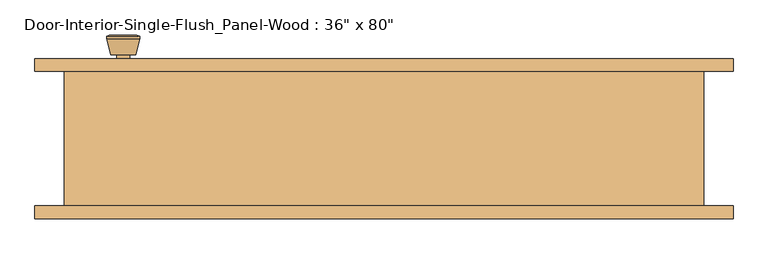
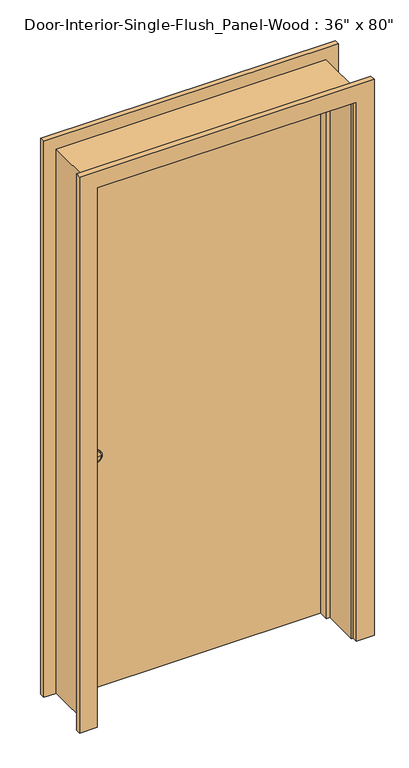
"""IFC4 building model written with IfcOpenShell, lengths in millimetres: door geometry."""

from ifc_helpers import new_model, si_unit, point, frame, frame_2d, origin, origin_with_axes, place, context, project, spatial, polyline, circle_curve, trimmed, segment, composite_curve, outline, extrude, faceted_brep, source, transform, mapped, element, save
from ifc_brep_helpers import plane_surface, cylinder_surface, revolved_surface, advanced_brep


def door_797b0c7a(model_context):
    return source(origin(), model_context, "Body", "SolidModel", [
        advanced_brep(
        [(-393.7, 57.5, 914.4), (-383.7, 57.5, 914.4), (-403.7, 57.5, 914.4), (-373.2241324, 8.5, 914.4), (-393.7, 8.5, 914.4), (-414.1758676, 8.5, 914.4), (-368.7, 10.3278681, 914.4), (-418.7, 10.3278681, 914.4), (-368.7, 13.7915463, 914.4), (-418.7, 13.7915463, 914.4), (-375.063764, 38.5, 914.4), (-412.336236, 38.5, 914.4), (-383.7, 38.5, 914.4), (-403.7, 38.5, 914.4)],
        [
            (0, 1),
            (1, 2, circle_curve(frame((-393.7, 57.5, 914.4), z_axis=(0.0, 1.0, 0.0), x_axis=(-1.0, 0.0, 0.0)), 10.0)),
            (2, 0),
            (2, 1, circle_curve(frame((-393.7, 57.5, 914.4), z_axis=(0.0, 1.0, 0.0), x_axis=(-1.0, 0.0, 0.0)), 10.0)),
            (3, 4),
            (4, 5),
            (5, 3, circle_curve(frame((-393.7, 8.5, 914.4), z_axis=(0.0, -1.0, 0.0), x_axis=(-1.0, 0.0, 0.0)), 20.4758676)),
            (3, 5, circle_curve(frame((-393.7, 8.5, 914.4), z_axis=(0.0, -1.0, 0.0), x_axis=(-1.0, 0.0, 0.0)), 20.4758676)),
            (6, 3),
            (5, 7),
            (7, 6, circle_curve(frame((-393.7, 10.3278681, 914.4), z_axis=(0.0, -1.0, 0.0), x_axis=(-1.0, 0.0, 0.0)), 25.0)),
            (6, 7, circle_curve(frame((-393.7, 10.3278681, 914.4), z_axis=(0.0, -1.0, 0.0), x_axis=(-1.0, 0.0, 0.0)), 25.0)),
            (8, 6),
            (7, 9),
            (9, 8, circle_curve(frame((-393.7, 13.7915463, 914.4), z_axis=(0.0, -1.0, 0.0), x_axis=(-1.0, 0.0, 0.0)), 25.0)),
            (8, 9, circle_curve(frame((-393.7, 13.7915463, 914.4), z_axis=(0.0, -1.0, 0.0), x_axis=(-1.0, 0.0, 0.0)), 25.0)),
            (10, 8),
            (9, 11),
            (11, 10, circle_curve(frame((-393.7, 38.5, 914.4), z_axis=(0.0, -1.0, 0.0), x_axis=(-1.0, 0.0, 0.0)), 18.636236)),
            (10, 11, circle_curve(frame((-393.7, 38.5, 914.4), z_axis=(0.0, -1.0, 0.0), x_axis=(-1.0, 0.0, 0.0)), 18.636236)),
            (12, 10),
            (11, 13),
            (13, 12, circle_curve(frame((-393.7, 38.5, 914.4), z_axis=(0.0, -1.0, 0.0), x_axis=(-1.0, 0.0, 0.0)), 10.0)),
            (12, 13, circle_curve(frame((-393.7, 38.5, 914.4), z_axis=(0.0, -1.0, 0.0), x_axis=(-1.0, 0.0, 0.0)), 10.0)),
            (1, 12),
            (13, 2),
        ],
        [
            plane_surface(frame((-393.7, 57.5, 914.4), z_axis=(0.0, 1.0, 0.0), x_axis=(-1.0, 0.0, 0.0))),
            plane_surface(frame((-393.7, 8.5, 914.4), z_axis=(0.0, -1.0, 0.0), x_axis=(-1.0, 0.0, 0.0))),
            revolved_surface(polyline([(-414.1758676, 8.5, 914.4), (-418.7, 10.3278681, 914.4)]), (-393.7, 57.5, 914.4), (0.0, 1.0, 0.0)),
            cylinder_surface(frame((-393.7, 57.5, 914.4), z_axis=(0.0, 1.0, 0.0), x_axis=(-1.0, 0.0, 0.0)), 25.0),
            revolved_surface(polyline([(-418.7, 13.7915463, 914.4), (-412.336236, 38.5, 914.4)]), (-393.7, 57.5, 914.4), (0.0, 1.0, 0.0)),
            plane_surface(frame((-393.7, 38.5, 914.4), z_axis=(0.0, 1.0, 0.0), x_axis=(-1.0, 0.0, 0.0))),
            cylinder_surface(frame((-393.7, 57.5, 914.4), z_axis=(0.0, 1.0, 0.0), x_axis=(-1.0, 0.0, 0.0)), 10.0),
        ],
        [
            (0, [[1, 2, 3]]),
            (0, [[-3, 4, -1]]),
            (1, [[5, 6, 7]]),
            (1, [[-6, -5, 8]]),
            (2, [[9, -7, 10, 11]]),
            (2, [[-10, -8, -9, 12]]),
            (3, [[13, -11, 14, 15]]),
            (3, [[-14, -12, -13, 16]]),
            (4, [[17, -15, 18, 19]]),
            (4, [[-18, -16, -17, 20]]),
            (5, [[21, -19, 22, 23]]),
            (5, [[-22, -20, -21, 24]]),
            (6, [[25, -23, 26, -2]]),
            (6, [[-26, -24, -25, -4]]),
        ],
    ),
        extrude(outline(composite_curve([segment(trimmed(circle_curve(frame_2d((914.4, -393.7)), 30.0), [point((914.4, -423.7))], [point((914.4, -363.7))], False, "CARTESIAN"), True, "CONTINUOUS"), segment(trimmed(circle_curve(frame_2d((914.4, -393.7)), 30.0), [point((914.4, -363.7))], [point((914.4, -423.7))], False, "CARTESIAN"), True, "CONTINUOUS")], self_intersect=False)), frame((0.0, 57.5, 0.0), z_axis=(0.0, 1.0, 0.0), x_axis=(0.0, 0.0, 1.0)), (0.0, 0.0, 1.0), 6.0),
        advanced_brep(
        [(-393.7, 104.425, 914.4), (-403.7, 104.425, 914.4), (-383.7, 104.425, 914.4), (-373.2241324, 153.425, 914.4), (-414.1758676, 153.425, 914.4), (-393.7, 153.425, 914.4), (-368.7, 151.5971319, 914.4), (-418.7, 151.5971319, 914.4), (-368.7, 148.1334537, 914.4), (-418.7, 148.1334537, 914.4), (-375.063764, 123.425, 914.4), (-412.336236, 123.425, 914.4), (-383.7, 123.425, 914.4), (-403.7, 123.425, 914.4)],
        [
            (0, 1),
            (1, 2, circle_curve(frame((-393.7, 104.425, 914.4), z_axis=(0.0, -1.0, 0.0), x_axis=(-1.0, 0.0, 0.0)), 10.0)),
            (2, 0),
            (2, 1, circle_curve(frame((-393.7, 104.425, 914.4), z_axis=(0.0, -1.0, 0.0), x_axis=(-1.0, 0.0, 0.0)), 10.0)),
            (3, 4, circle_curve(frame((-393.7, 153.425, 914.4), z_axis=(0.0, 1.0, 0.0), x_axis=(-1.0, 0.0, 0.0)), 20.4758676)),
            (4, 5),
            (5, 3),
            (4, 3, circle_curve(frame((-393.7, 153.425, 914.4), z_axis=(0.0, 1.0, 0.0), x_axis=(-1.0, 0.0, 0.0)), 20.4758676)),
            (6, 7, circle_curve(frame((-393.7, 151.5971319, 914.4), z_axis=(0.0, 1.0, 0.0), x_axis=(-1.0, 0.0, 0.0)), 25.0)),
            (7, 4),
            (3, 6),
            (7, 6, circle_curve(frame((-393.7, 151.5971319, 914.4), z_axis=(0.0, 1.0, 0.0), x_axis=(-1.0, 0.0, 0.0)), 25.0)),
            (8, 9, circle_curve(frame((-393.7, 148.1334537, 914.4), z_axis=(0.0, 1.0, 0.0), x_axis=(-1.0, 0.0, 0.0)), 25.0)),
            (9, 7),
            (6, 8),
            (9, 8, circle_curve(frame((-393.7, 148.1334537, 914.4), z_axis=(0.0, 1.0, 0.0), x_axis=(-1.0, 0.0, 0.0)), 25.0)),
            (10, 11, circle_curve(frame((-393.7, 123.425, 914.4), z_axis=(0.0, 1.0, 0.0), x_axis=(-1.0, 0.0, 0.0)), 18.636236)),
            (11, 9),
            (8, 10),
            (11, 10, circle_curve(frame((-393.7, 123.425, 914.4), z_axis=(0.0, 1.0, 0.0), x_axis=(-1.0, 0.0, 0.0)), 18.636236)),
            (12, 13, circle_curve(frame((-393.7, 123.425, 914.4), z_axis=(0.0, 1.0, 0.0), x_axis=(-1.0, 0.0, 0.0)), 10.0)),
            (13, 11),
            (10, 12),
            (13, 12, circle_curve(frame((-393.7, 123.425, 914.4), z_axis=(0.0, 1.0, 0.0), x_axis=(-1.0, 0.0, 0.0)), 10.0)),
            (1, 13),
            (12, 2),
        ],
        [
            plane_surface(frame((-393.7, 104.425, 914.4), z_axis=(0.0, -1.0, 0.0), x_axis=(-1.0, 0.0, 0.0))),
            plane_surface(frame((-393.7, 153.425, 914.4), z_axis=(0.0, 1.0, 0.0), x_axis=(-1.0, 0.0, 0.0))),
            revolved_surface(polyline([(-414.1758676, 153.425, 914.4), (-418.7, 151.5971319, 914.4)]), (-393.7, 104.425, 914.4), (0.0, -1.0, 0.0)),
            cylinder_surface(frame((-393.7, 104.425, 914.4), z_axis=(0.0, -1.0, 0.0), x_axis=(-1.0, 0.0, 0.0)), 25.0),
            revolved_surface(polyline([(-418.7, 148.1334537, 914.4), (-412.336236, 123.425, 914.4)]), (-393.7, 104.425, 914.4), (0.0, -1.0, 0.0)),
            plane_surface(frame((-393.7, 123.425, 914.4), z_axis=(0.0, -1.0, 0.0), x_axis=(-1.0, 0.0, 0.0))),
            cylinder_surface(frame((-393.7, 104.425, 914.4), z_axis=(0.0, -1.0, 0.0), x_axis=(-1.0, 0.0, 0.0)), 10.0),
        ],
        [
            (0, [[1, 2, 3]]),
            (0, [[-3, 4, -1]]),
            (1, [[5, 6, 7]]),
            (1, [[8, -7, -6]]),
            (2, [[9, 10, -5, 11]]),
            (2, [[12, -11, -8, -10]]),
            (3, [[13, 14, -9, 15]]),
            (3, [[16, -15, -12, -14]]),
            (4, [[17, 18, -13, 19]]),
            (4, [[20, -19, -16, -18]]),
            (5, [[21, 22, -17, 23]]),
            (5, [[24, -23, -20, -22]]),
            (6, [[-2, 25, -21, 26]]),
            (6, [[-4, -26, -24, -25]]),
        ],
    ),
        extrude(outline(composite_curve([segment(trimmed(circle_curve(frame_2d((914.4, -393.7)), 30.0), [point((914.4, -423.7))], [point((914.4, -363.7))], False, "CARTESIAN"), True, "CONTINUOUS"), segment(trimmed(circle_curve(frame_2d((914.4, -393.7)), 30.0), [point((914.4, -363.7))], [point((914.4, -423.7))], False, "CARTESIAN"), True, "CONTINUOUS")], self_intersect=False)), frame((0.0, 98.425, 0.0), z_axis=(0.0, 1.0, 0.0), x_axis=(0.0, 0.0, 1.0)), (0.0, 0.0, 1.0), 6.0),
        extrude(outline(polyline([(457.2, 63.5), (-457.2, 63.5), (-457.2, 98.425), (457.2, 98.425), (457.2, 63.5)])), origin_with_axes(), (0.0, 0.0, 1.0), 2032.0),
        faceted_brep([(482.6, 98.425, 0.0), (482.6, -104.775, 0.0), (457.2, -104.775, 0.0), (457.2, 28.575, 0.0), (444.5, 28.575, 0.0), (444.5, 63.5, 0.0), (457.2, 63.5, 0.0), (457.2, 98.425, 0.0), (482.6, 98.425, 2057.4), (482.6, -104.775, 2057.4), (-482.6, -104.775, 2057.4), (-482.6, -104.775, 0.0), (-457.2, -104.775, 0.0), (-457.2, -104.775, 2032.0), (457.2, -104.775, 2032.0), (457.2, 28.575, 2032.0), (-457.2, 28.575, 2032.0), (-457.2, 28.575, 0.0), (-444.5, 28.575, 0.0), (-444.5, 28.575, 2019.3), (444.5, 28.575, 2019.3), (444.5, 63.5, 2019.3), (-444.5, 63.5, 2019.3), (-444.5, 63.5, 0.0), (-457.2, 63.5, 0.0), (-457.2, 63.5, 2032.0), (457.2, 63.5, 2032.0), (457.2, 98.425, 2032.0), (-457.2, 98.425, 2032.0), (-457.2, 98.425, 0.0), (-482.6, 98.425, 0.0), (-482.6, 98.425, 2057.4)], [[[0, 1, 2, 3, 4, 5, 6, 7]], [[1, 0, 8, 9]], [[2, 1, 9, 10, 11, 12, 13, 14]], [[3, 2, 14, 15]], [[4, 3, 15, 16, 17, 18, 19, 20]], [[5, 4, 20, 21]], [[6, 5, 21, 22, 23, 24, 25, 26]], [[7, 6, 26, 27]], [[0, 7, 27, 28, 29, 30, 31, 8]], [[9, 8, 31, 10]], [[15, 14, 13, 16]], [[21, 20, 19, 22]], [[27, 26, 25, 28]], [[30, 29, 24, 23, 18, 17, 12, 11]], [[10, 31, 30, 11]], [[16, 13, 12, 17]], [[22, 19, 18, 23]], [[28, 25, 24, 29]]]),
        extrude(outline(polyline([(0.0, 463.55), (0.0, 527.05), (2101.85, 527.05), (2101.85, -527.05), (0.0, -527.05), (0.0, -463.55), (2038.35, -463.55), (2038.35, 463.55), (0.0, 463.55)])), frame((0.0, -123.825, 0.0), z_axis=(0.0, 1.0, 0.0), x_axis=(0.0, 0.0, 1.0)), (0.0, 0.0, 1.0), 19.05),
        extrude(outline(polyline([(0.0, 463.55), (0.0, 527.05), (2101.85, 527.05), (2101.85, -527.05), (0.0, -527.05), (0.0, -463.55), (2038.35, -463.55), (2038.35, 463.55), (0.0, 463.55)])), frame((0.0, 98.425, 0.0), z_axis=(0.0, 1.0, 0.0), x_axis=(0.0, 0.0, 1.0)), (0.0, 0.0, 1.0), 19.05),
    ])


if __name__ == "__main__":
    model = new_model("IFC4")
    model_context = context("Model", 3, world=origin())
    ifc_project = project(units=[si_unit("LENGTHUNIT", "METRE", prefix="MILLI")], contexts=[model_context])
    site = spatial("IfcSite", under=ifc_project)
    building = spatial("IfcBuilding", under=site)
    placement = place(None, origin())
    door_shape = door_797b0c7a(model_context)
    element("IfcDoor", 1, ObjectType="Door-Interior-Single-Flush_Panel-Wood : 36\" x 80\"", at=placement, inside=building, context=model_context, shape_type="MappedRepresentation", body=[
        mapped(door_shape, transform((0.0, 0.0, 0.0), x_axis=(1.0, 0.0, 0.0), y_axis=(0.0, 1.0, 0.0), z_axis=(0.0, 0.0, 1.0))),
    ])
    save(model, "model.ifc")

# Revit data of these elements
# Type "Door-Interior-Single-Flush_Panel-Wood : 36\" x 80\""
#   Type Mark = "17"
#   Assembly Code = "C1020300"
#   Analytic Construction = "Wooden"
#   Thickness = 0' - 1 3/8"
#   Thermal Resistance (R) = 2.5876 (h·ft²·°F)/BTU
#   Swing Angle [instance default] = 90.00°
#   Rough Width = 3' - 2"
#   Rough Height = 6' - 9"
#   Height = 6' - 8"
#   Width = 3' - 0"
#   Heat Transfer Coefficient (U) = 0.3865 BTU/(h·ft²·°F)
#   Trim Material = Cherry
#   Panel Material = Cherry
#   Frame Material = Cherry
#   Door Handle Material = Aluminum
#   Visual Light Transmittance = 0
#   Solar Heat Gain Coefficient = 0
#   Wall Closure = (empty or 0)
#   Function = (empty or 0)
# Element 1 (IfcDoor, "Door-Interior-Single-Flush_Panel-Wood : 36\" x 80\"")
#   Materials on its faces: "Cherry", "Aluminum"
# Materials
#   "Cherry": class "Wood", colour RGB 226 177 128, transparency 0, Description = "Prunus Serotina", Cost = 0
#   "Aluminum": class "Metal", colour RGB 247 247 247, transparency 0, Description = "Aluminum 6061", Cost = 0
